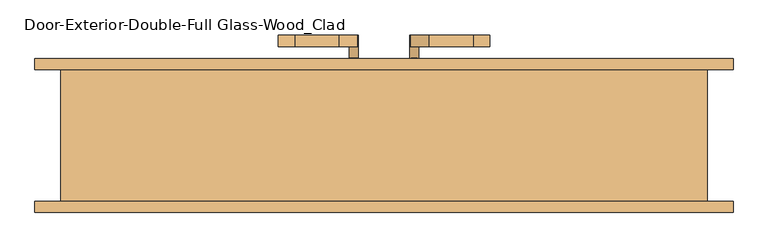
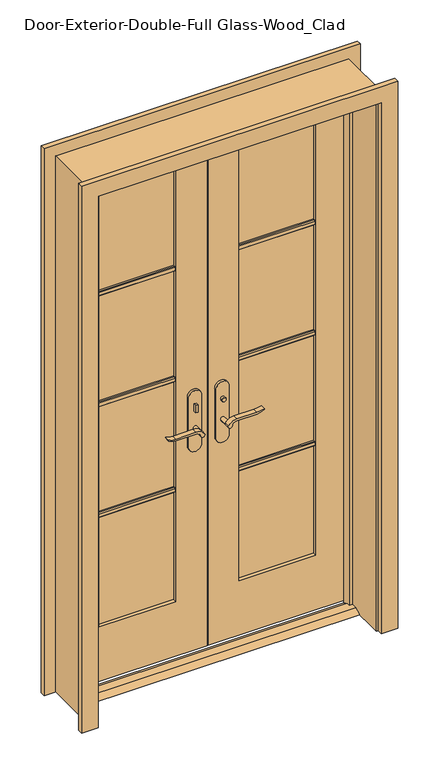
"""IFC4 building model written with IfcOpenShell, lengths in millimetres: door geometry, Door-Exterior-Double-Full Glass-Wood_Clad."""

from ifc_helpers import new_model, si_unit, point, frame, frame_2d, origin, place, context, project, spatial, polyline, circle_curve, trimmed, segment, composite_curve, outline, extrude, faceted_brep, source, transform, mapped, element, save


def door_exterior_double_full_glass_wood_clad_a9b2ee3b(model_context):
    return source(origin(), model_context, "Body", "SolidModel", [
        extrude(outline(polyline([(19.05, 12.7), (53.975, 12.7), (79.375, 0.0), (-6.35, 0.0), (19.05, 12.7)])), frame((-533.4, 0.0, 0.0), z_axis=(1.0, 0.0, 0.0), x_axis=(0.0, 1.0, 0.0)), (0.0, 0.0, 1.0), 1066.8),
        extrude(outline(polyline([(-47.4019111, 56.2), (-57.4019111, 56.2), (-57.4019111, 66.2), (-47.4019111, 66.2), (-47.4019111, 56.2)])), frame((0.0, 0.0, 981.9), z_axis=(0.0, 0.0, 1.0), x_axis=(1.0, 0.0, 0.0)), (0.0, 0.0, 1.0), 30.0),
        extrude(outline(composite_curve([segment(trimmed(circle_curve(frame_2d((996.9, -52.4019111)), 8.0), [point((996.9, -60.4019111))], [point((996.9, -44.4019111))], False, "CARTESIAN"), True, "CONTINUOUS"), segment(trimmed(circle_curve(frame_2d((996.9, -52.4019111)), 8.0), [point((996.9, -44.4019111))], [point((996.9, -60.4019111))], False, "CARTESIAN"), True, "CONTINUOUS")], self_intersect=False)), frame((0.0, 121.125, 0.0), z_axis=(0.0, 1.0, 0.0), x_axis=(0.0, 0.0, 1.0)), (0.0, 0.0, 1.0), 10.0),
        extrude(outline(composite_curve([segment(trimmed(circle_curve(frame_2d((897.1555521, -76.0694241)), 37.2832219), [point((919.0523287, -45.8937749))], [point((934.4, -77.7693445))], False, "CARTESIAN"), True, "CONTINUOUS"), segment(polyline([(934.4, -77.7693445), (934.4, -154.045502)]), True, "CONTINUOUS"), segment(trimmed(circle_curve(frame_2d((1017.6850638, -153.9791202)), 83.2850902), [point((934.4, -154.045502))], [point((939.4, -182.4019111))], True, "CARTESIAN"), True, "CONTINUOUS"), segment(polyline([(939.4, -182.4019111), (936.6135558, -182.4019111)]), True, "CONTINUOUS"), segment(trimmed(circle_curve(frame_2d((986.6709207, -150.4622499)), 59.3791355), [point((936.6135558, -182.4019111))], [point((927.4, -154.045502))], False, "CARTESIAN"), True, "CONTINUOUS"), segment(polyline([(927.4, -154.045502), (927.4, -77.7881013)]), True, "CONTINUOUS"), segment(trimmed(circle_curve(frame_2d((909.2738613, -77.7881013)), 18.1261387), [point((927.4, -77.7881013))], [point((914.4, -60.4019111))], True, "CARTESIAN"), True, "CONTINUOUS"), segment(trimmed(circle_curve(frame_2d((914.4, -52.4019111)), 8.0), [point((914.4, -60.4019111))], [point((919.0523287, -45.8937749))], False, "CARTESIAN"), True, "CONTINUOUS")], self_intersect=False)), frame((0.0, 16.2, 0.0), z_axis=(0.0, 1.0, 0.0), x_axis=(0.0, 0.0, 1.0)), (0.0, 0.0, 1.0), 20.0),
        extrude(outline(composite_curve([segment(trimmed(circle_curve(frame_2d((914.4, -52.4019111)), 8.0), [point((914.3999903, -60.4019111))], [point((919.0523287, -45.8937749))], False, "CARTESIAN"), True, "CONTINUOUS"), segment(trimmed(circle_curve(frame_2d((897.1555521, -76.0694241)), 37.2832219), [point((919.0523287, -45.8937749))], [point((934.4, -77.7693445))], False, "CARTESIAN"), True, "CONTINUOUS"), segment(polyline([(934.4, -77.7693445), (934.4, -154.045502)]), True, "CONTINUOUS"), segment(trimmed(circle_curve(frame_2d((1017.6850638, -153.9791202)), 83.2850902), [point((934.4, -154.045502))], [point((939.4, -182.4019111))], True, "CARTESIAN"), True, "CONTINUOUS"), segment(polyline([(939.4, -182.4019111), (936.6135558, -182.4019111)]), True, "CONTINUOUS"), segment(trimmed(circle_curve(frame_2d((986.6709207, -150.4622499)), 59.3791355), [point((936.6135558, -182.4019111))], [point((927.4, -154.045502))], False, "CARTESIAN"), True, "CONTINUOUS"), segment(polyline([(927.4, -154.045502), (927.4, -77.788099)]), True, "CONTINUOUS"), segment(trimmed(circle_curve(frame_2d((909.2738682, -77.788099)), 18.1261318), [point((927.4, -77.788099))], [point((914.3999903, -60.4019111))], True, "CARTESIAN"), True, "CONTINUOUS")], self_intersect=False)), frame((0.0, 151.125, 0.0), z_axis=(0.0, 1.0, 0.0), x_axis=(0.0, 0.0, 1.0)), (0.0, 0.0, 1.0), 20.0),
        extrude(outline(composite_curve([segment(trimmed(circle_curve(frame_2d((914.4, -52.4019111)), 8.0), [point((914.4, -60.4019111))], [point((914.4, -44.4019111))], False, "CARTESIAN"), True, "CONTINUOUS"), segment(trimmed(circle_curve(frame_2d((914.4, -52.4019111)), 8.0), [point((914.4, -44.4019111))], [point((914.4, -60.4019111))], False, "CARTESIAN"), True, "CONTINUOUS")], self_intersect=False)), frame((0.0, 36.2, 0.0), z_axis=(0.0, 1.0, 0.0), x_axis=(0.0, 0.0, 1.0)), (0.0, 0.0, 1.0), 30.0),
        extrude(outline(composite_curve([segment(trimmed(circle_curve(frame_2d((914.4, -52.4019111)), 8.0), [point((914.4, -60.4019111))], [point((914.4, -44.4019111))], False, "CARTESIAN"), True, "CONTINUOUS"), segment(trimmed(circle_curve(frame_2d((914.4, -52.4019111)), 8.0), [point((914.4, -44.4019111))], [point((914.4, -60.4019111))], False, "CARTESIAN"), True, "CONTINUOUS")], self_intersect=False)), frame((0.0, 121.125, 0.0), z_axis=(0.0, 1.0, 0.0), x_axis=(0.0, 0.0, 1.0)), (0.0, 0.0, 1.0), 30.0),
        extrude(outline(composite_curve([segment(polyline([(844.4, -27.4019111), (1039.4, -27.4019111)]), True, "CONTINUOUS"), segment(trimmed(circle_curve(frame_2d((1039.4, -52.4019111)), 25.0), [point((1039.4, -27.4019111))], [point((1039.4, -77.4019111))], False, "CARTESIAN"), True, "CONTINUOUS"), segment(polyline([(1039.4, -77.4019111), (844.4, -77.4019111)]), True, "CONTINUOUS"), segment(trimmed(circle_curve(frame_2d((844.4, -52.4019111)), 25.0), [point((844.4, -77.4019111))], [point((844.4, -27.4019111))], False, "CARTESIAN"), True, "CONTINUOUS")], self_intersect=False)), frame((0.0, 66.2, 0.0), z_axis=(0.0, 1.0, 0.0), x_axis=(0.0, 0.0, 1.0)), (0.0, 0.0, 1.0), 10.0),
        extrude(outline(composite_curve([segment(polyline([(844.4, -27.4019111), (1039.4, -27.4019111)]), True, "CONTINUOUS"), segment(trimmed(circle_curve(frame_2d((1039.4, -52.4019111)), 25.0), [point((1039.4, -27.4019111))], [point((1039.4, -77.4019111))], False, "CARTESIAN"), True, "CONTINUOUS"), segment(polyline([(1039.4, -77.4019111), (844.4, -77.4019111)]), True, "CONTINUOUS"), segment(trimmed(circle_curve(frame_2d((844.4, -52.4019111)), 25.0), [point((844.4, -77.4019111))], [point((844.4, -27.4019111))], False, "CARTESIAN"), True, "CONTINUOUS")], self_intersect=False)), frame((0.0, 111.125, 0.0), z_axis=(0.0, 1.0, 0.0), x_axis=(0.0, 0.0, 1.0)), (0.0, 0.0, 1.0), 10.0),
        extrude(outline(polyline([(47.3875, 131.125), (57.3875, 131.125), (57.3875, 121.125), (47.3875, 121.125), (47.3875, 131.125)])), frame((0.0, 0.0, 981.9), z_axis=(0.0, 0.0, 1.0), x_axis=(1.0, 0.0, 0.0)), (0.0, 0.0, 1.0), 30.0),
        extrude(outline(composite_curve([segment(trimmed(circle_curve(frame_2d((996.9, 52.3875)), 8.0), [point((996.9, 60.3875))], [point((996.9, 44.3875))], False, "CARTESIAN"), True, "CONTINUOUS"), segment(trimmed(circle_curve(frame_2d((996.9, 52.3875)), 8.0), [point((996.9, 44.3875))], [point((996.9, 60.3875))], False, "CARTESIAN"), True, "CONTINUOUS")], self_intersect=False)), frame((0.0, 56.2, 0.0), z_axis=(0.0, 1.0, 0.0), x_axis=(0.0, 0.0, 1.0)), (0.0, 0.0, 1.0), 10.0),
        extrude(outline(composite_curve([segment(trimmed(circle_curve(frame_2d((914.4, 52.3875)), 8.0), [point((919.0523287, 45.8793637))], [point((914.4, 60.3875))], False, "CARTESIAN"), True, "CONTINUOUS"), segment(trimmed(circle_curve(frame_2d((909.2738613, 77.7736901)), 18.1261387), [point((914.4, 60.3875))], [point((927.4, 77.7736901))], True, "CARTESIAN"), True, "CONTINUOUS"), segment(polyline([(927.4, 77.7736901), (927.4, 154.0310909)]), True, "CONTINUOUS"), segment(trimmed(circle_curve(frame_2d((986.6709207, 150.4478388)), 59.3791355), [point((927.4, 154.0310909))], [point((936.6135558, 182.3875))], False, "CARTESIAN"), True, "CONTINUOUS"), segment(polyline([(936.6135558, 182.3875), (939.4, 182.3875)]), True, "CONTINUOUS"), segment(trimmed(circle_curve(frame_2d((1017.6850638, 153.9647091)), 83.2850902), [point((939.4, 182.3875))], [point((934.4, 154.0310909))], True, "CARTESIAN"), True, "CONTINUOUS"), segment(polyline([(934.4, 154.0310909), (934.4, 77.7549333)]), True, "CONTINUOUS"), segment(trimmed(circle_curve(frame_2d((897.1555521, 76.0550129)), 37.2832219), [point((934.4, 77.7549333))], [point((919.0523287, 45.8793637))], False, "CARTESIAN"), True, "CONTINUOUS")], self_intersect=False)), frame((0.0, 151.125, 0.0), z_axis=(0.0, 1.0, 0.0), x_axis=(0.0, 0.0, 1.0)), (0.0, 0.0, 1.0), 20.0),
        extrude(outline(composite_curve([segment(trimmed(circle_curve(frame_2d((909.2738682, 77.7736878)), 18.1261318), [point((914.3999903, 60.3875))], [point((927.4, 77.7736878))], True, "CARTESIAN"), True, "CONTINUOUS"), segment(polyline([(927.4, 77.7736878), (927.4, 154.0310909)]), True, "CONTINUOUS"), segment(trimmed(circle_curve(frame_2d((986.6709207, 150.4478388)), 59.3791355), [point((927.4, 154.0310909))], [point((936.6135558, 182.3875))], False, "CARTESIAN"), True, "CONTINUOUS"), segment(polyline([(936.6135558, 182.3875), (939.4, 182.3875)]), True, "CONTINUOUS"), segment(trimmed(circle_curve(frame_2d((1017.6850638, 153.9647091)), 83.2850902), [point((939.4, 182.3875))], [point((934.4, 154.0310909))], True, "CARTESIAN"), True, "CONTINUOUS"), segment(polyline([(934.4, 154.0310909), (934.4, 77.7549333)]), True, "CONTINUOUS"), segment(trimmed(circle_curve(frame_2d((897.1555521, 76.0550129)), 37.2832219), [point((934.4, 77.7549333))], [point((919.0523287, 45.8793637))], False, "CARTESIAN"), True, "CONTINUOUS"), segment(trimmed(circle_curve(frame_2d((914.4, 52.3875)), 8.0), [point((919.0523287, 45.8793637))], [point((914.3999903, 60.3875))], False, "CARTESIAN"), True, "CONTINUOUS")], self_intersect=False)), frame((0.0, 16.2, 0.0), z_axis=(0.0, 1.0, 0.0), x_axis=(0.0, 0.0, 1.0)), (0.0, 0.0, 1.0), 20.0),
        extrude(outline(composite_curve([segment(trimmed(circle_curve(frame_2d((914.4, 52.3875)), 8.0), [point((914.4, 60.3875))], [point((914.4, 44.3875))], False, "CARTESIAN"), True, "CONTINUOUS"), segment(trimmed(circle_curve(frame_2d((914.4, 52.3875)), 8.0), [point((914.4, 44.3875))], [point((914.4, 60.3875))], False, "CARTESIAN"), True, "CONTINUOUS")], self_intersect=False)), frame((0.0, 121.125, 0.0), z_axis=(0.0, 1.0, 0.0), x_axis=(0.0, 0.0, 1.0)), (0.0, 0.0, 1.0), 30.0),
        extrude(outline(composite_curve([segment(trimmed(circle_curve(frame_2d((914.4, 52.3875)), 8.0), [point((914.4, 60.3875))], [point((914.4, 44.3875))], False, "CARTESIAN"), True, "CONTINUOUS"), segment(trimmed(circle_curve(frame_2d((914.4, 52.3875)), 8.0), [point((914.4, 44.3875))], [point((914.4, 60.3875))], False, "CARTESIAN"), True, "CONTINUOUS")], self_intersect=False)), frame((0.0, 36.2, 0.0), z_axis=(0.0, 1.0, 0.0), x_axis=(0.0, 0.0, 1.0)), (0.0, 0.0, 1.0), 30.0),
        extrude(outline(composite_curve([segment(trimmed(circle_curve(frame_2d((844.4, 52.3875)), 25.0), [point((844.4, 27.3875))], [point((844.4, 77.3875))], False, "CARTESIAN"), True, "CONTINUOUS"), segment(polyline([(844.4, 77.3875), (1039.4, 77.3875)]), True, "CONTINUOUS"), segment(trimmed(circle_curve(frame_2d((1039.4, 52.3875)), 25.0), [point((1039.4, 77.3875))], [point((1039.4, 27.3875))], False, "CARTESIAN"), True, "CONTINUOUS"), segment(polyline([(1039.4, 27.3875), (844.4, 27.3875)]), True, "CONTINUOUS")], self_intersect=False)), frame((0.0, 111.125, 0.0), z_axis=(0.0, 1.0, 0.0), x_axis=(0.0, 0.0, 1.0)), (0.0, 0.0, 1.0), 10.0),
        extrude(outline(composite_curve([segment(trimmed(circle_curve(frame_2d((844.4, 52.3875)), 25.0), [point((844.4, 27.3875))], [point((844.4, 77.3875))], False, "CARTESIAN"), True, "CONTINUOUS"), segment(polyline([(844.4, 77.3875), (1039.4, 77.3875)]), True, "CONTINUOUS"), segment(trimmed(circle_curve(frame_2d((1039.4, 52.3875)), 25.0), [point((1039.4, 77.3875))], [point((1039.4, 27.3875))], False, "CARTESIAN"), True, "CONTINUOUS"), segment(polyline([(1039.4, 27.3875), (844.4, 27.3875)]), True, "CONTINUOUS")], self_intersect=False)), frame((0.0, 66.2, 0.0), z_axis=(0.0, 1.0, 0.0), x_axis=(0.0, 0.0, 1.0)), (0.0, 0.0, 1.0), 10.0),
        extrude(outline(polyline([(90.17, 1578.371875), (90.17, 1559.321875), (83.82, 1559.321875), (80.645, 1562.496875), (80.645, 1575.196875), (83.82, 1578.371875), (90.17, 1578.371875)])), frame((120.65, 0.0, 0.0), z_axis=(1.0, 0.0, 0.0), x_axis=(0.0, 1.0, 0.0)), (0.0, 0.0, 1.0), 292.1),
        extrude(outline(polyline([(90.17, 1132.68125), (90.17, 1113.63125), (83.82, 1113.63125), (80.645, 1116.80625), (80.645, 1129.50625), (83.82, 1132.68125), (90.17, 1132.68125)])), frame((120.65, 0.0, 0.0), z_axis=(1.0, 0.0, 0.0), x_axis=(0.0, 1.0, 0.0)), (0.0, 0.0, 1.0), 292.1),
        extrude(outline(polyline([(90.17, 686.990625), (90.17, 667.940625), (83.82, 667.940625), (80.645, 671.115625), (80.645, 683.815625), (83.82, 686.990625), (90.17, 686.990625)])), frame((120.65, 0.0, 0.0), z_axis=(1.0, 0.0, 0.0), x_axis=(0.0, 1.0, 0.0)), (0.0, 0.0, 1.0), 292.1),
        extrude(outline(polyline([(97.155, 1578.371875), (103.505, 1578.371875), (106.68, 1575.196875), (106.68, 1562.496875), (103.505, 1559.321875), (97.155, 1559.321875), (97.155, 1578.371875)])), frame((-412.75, 0.0, 0.0), z_axis=(1.0, 0.0, 0.0), x_axis=(0.0, 1.0, 0.0)), (0.0, 0.0, 1.0), 292.1),
        extrude(outline(polyline([(97.155, 1132.68125), (103.505, 1132.68125), (106.68, 1129.50625), (106.68, 1116.80625), (103.505, 1113.63125), (97.155, 1113.63125), (97.155, 1132.68125)])), frame((-412.75, 0.0, 0.0), z_axis=(1.0, 0.0, 0.0), x_axis=(0.0, 1.0, 0.0)), (0.0, 0.0, 1.0), 292.1),
        extrude(outline(polyline([(97.155, 686.990625), (103.505, 686.990625), (106.68, 683.815625), (106.68, 671.115625), (103.505, 667.940625), (97.155, 667.940625), (97.155, 686.990625)])), frame((-412.75, 0.0, 0.0), z_axis=(1.0, 0.0, 0.0), x_axis=(0.0, 1.0, 0.0)), (0.0, 0.0, 1.0), 292.1),
        extrude(outline(polyline([(97.155, 1578.371875), (103.505, 1578.371875), (106.68, 1575.196875), (106.68, 1562.496875), (103.505, 1559.321875), (97.155, 1559.321875), (97.155, 1578.371875)])), frame((120.65, 0.0, 0.0), z_axis=(1.0, 0.0, 0.0), x_axis=(0.0, 1.0, 0.0)), (0.0, 0.0, 1.0), 292.1),
        extrude(outline(polyline([(97.155, 1132.68125), (103.505, 1132.68125), (106.68, 1129.50625), (106.68, 1116.80625), (103.505, 1113.63125), (97.155, 1113.63125), (97.155, 1132.68125)])), frame((120.65, 0.0, 0.0), z_axis=(1.0, 0.0, 0.0), x_axis=(0.0, 1.0, 0.0)), (0.0, 0.0, 1.0), 292.1),
        extrude(outline(polyline([(97.155, 686.990625), (103.505, 686.990625), (106.68, 683.815625), (106.68, 671.115625), (103.505, 667.940625), (97.155, 667.940625), (97.155, 686.990625)])), frame((120.65, 0.0, 0.0), z_axis=(1.0, 0.0, 0.0), x_axis=(0.0, 1.0, 0.0)), (0.0, 0.0, 1.0), 292.1),
        extrude(outline(polyline([(90.17, 1578.371875), (90.17, 1559.321875), (83.82, 1559.321875), (80.645, 1562.496875), (80.645, 1575.196875), (83.82, 1578.371875), (90.17, 1578.371875)])), frame((-412.75, 0.0, 0.0), z_axis=(1.0, 0.0, 0.0), x_axis=(0.0, 1.0, 0.0)), (0.0, 0.0, 1.0), 292.1),
        extrude(outline(polyline([(90.17, 1132.68125), (90.17, 1113.63125), (83.82, 1113.63125), (80.645, 1116.80625), (80.645, 1129.50625), (83.82, 1132.68125), (90.17, 1132.68125)])), frame((-412.75, 0.0, 0.0), z_axis=(1.0, 0.0, 0.0), x_axis=(0.0, 1.0, 0.0)), (0.0, 0.0, 1.0), 292.1),
        extrude(outline(polyline([(90.17, 686.990625), (90.17, 667.940625), (83.82, 667.940625), (80.645, 671.115625), (80.645, 683.815625), (83.82, 686.990625), (90.17, 686.990625)])), frame((-412.75, 0.0, 0.0), z_axis=(1.0, 0.0, 0.0), x_axis=(0.0, 1.0, 0.0)), (0.0, 0.0, 1.0), 292.1),
        extrude(outline(polyline([(0.0, 539.75), (0.0, 603.25), (2203.45, 603.25), (2203.45, -603.25), (0.0, -603.25), (0.0, -539.75), (2139.95, -539.75), (2139.95, 539.75), (0.0, 539.75)])), frame((0.0, -136.525, 0.0), z_axis=(0.0, 1.0, 0.0), x_axis=(0.0, 0.0, 1.0)), (0.0, 0.0, 1.0), 19.05),
        extrude(outline(polyline([(0.0, 539.75), (0.0, 603.25), (2203.45, 603.25), (2203.45, -603.25), (0.0, -603.25), (0.0, -539.75), (2139.95, -539.75), (2139.95, 539.75), (0.0, 539.75)])), frame((0.0, 111.125, 0.0), z_axis=(0.0, 1.0, 0.0), x_axis=(0.0, 0.0, 1.0)), (0.0, 0.0, 1.0), 19.05),
        faceted_brep([(558.8, 111.125, 0.0), (558.8, -117.475, 0.0), (533.4, -117.475, 0.0), (533.4, 41.275, 0.0), (520.7, 41.275, 0.0), (520.7, 76.2, 0.0), (533.4, 76.2, 0.0), (533.4, 111.125, 0.0), (558.8, 111.125, 2159.0), (558.8, -117.475, 2159.0), (-558.8, -117.475, 2159.0), (-558.8, -117.475, 0.0), (-533.4, -117.475, 0.0), (-533.4, -117.475, 2133.6), (533.4, -117.475, 2133.6), (533.4, 41.275, 2133.6), (-533.4, 41.275, 2133.6), (-533.4, 41.275, 0.0), (-520.7, 41.275, 0.0), (-520.7, 41.275, 2120.9), (520.7, 41.275, 2120.9), (520.7, 76.2, 2120.9), (1.5875, 76.2, 2120.9), (-1.6019111, 76.2, 2120.9), (-520.7, 76.2, 2120.9), (-520.7, 76.2, 0.0), (-533.4, 76.2, 0.0), (-533.4, 76.2, 2133.6), (-1.6019111, 76.2, 2133.6), (1.5875, 76.2, 2133.6), (533.4, 76.2, 2133.6), (533.4, 111.125, 2133.6), (1.5875, 111.125, 2133.6), (-1.6019111, 111.125, 2133.6), (-533.4, 111.125, 2133.6), (-533.4, 111.125, 0.0), (-558.8, 111.125, 0.0), (-558.8, 111.125, 2159.0)], [[[0, 1, 2, 3, 4, 5, 6, 7]], [[1, 0, 8, 9]], [[2, 1, 9, 10, 11, 12, 13, 14]], [[3, 2, 14, 15]], [[4, 3, 15, 16, 17, 18, 19, 20]], [[5, 4, 20, 21]], [[6, 5, 21, 22, 23, 24, 25, 26, 27, 28, 29, 30]], [[7, 6, 30, 31]], [[0, 7, 31, 32, 33, 34, 35, 36, 37, 8]], [[9, 8, 37, 10]], [[14, 13, 16, 15]], [[20, 19, 24, 23, 22, 21]], [[31, 30, 29, 28, 27, 34, 33, 32]], [[12, 11, 36, 35, 26, 25, 18, 17]], [[11, 10, 37, 36]], [[13, 12, 17, 16]], [[19, 18, 25, 24]], [[27, 26, 35, 34]]]),
        extrude(outline(polyline([(12.7, 533.4), (2133.6, 533.4), (2133.6, 1.5875), (12.7, 1.5875), (12.7, 533.4)]), holes=[polyline([(2014.5375, 120.65), (2014.5375, 412.75), (231.775, 412.75), (231.775, 120.65), (2014.5375, 120.65)])]), frame((0.0, 76.2, 0.0), z_axis=(0.0, 1.0, 0.0), x_axis=(0.0, 0.0, 1.0)), (0.0, 0.0, 1.0), 34.925),
        extrude(outline(polyline([(2133.6, -533.4), (12.7, -533.4), (12.7, -1.6019111), (2133.6, -1.6019111), (2133.6, -533.4)]), holes=[polyline([(231.775, -412.75), (2014.5375, -412.75), (2014.5375, -120.65), (231.775, -120.65), (231.775, -412.75)])]), frame((0.0, 76.2, 0.0), z_axis=(0.0, 1.0, 0.0), x_axis=(0.0, 0.0, 1.0)), (0.0, 0.0, 1.0), 34.925),
        extrude(outline(polyline([(412.75, 90.17), (120.65, 90.17), (120.65, 97.155), (412.75, 97.155), (412.75, 90.17)])), frame((0.0, 0.0, 231.775), z_axis=(0.0, 0.0, 1.0), x_axis=(1.0, 0.0, 0.0)), (0.0, 0.0, 1.0), 1782.7625),
        extrude(outline(polyline([(-120.65, 90.17), (-412.75, 90.17), (-412.75, 97.155), (-120.65, 97.155), (-120.65, 90.17)])), frame((0.0, 0.0, 231.775), z_axis=(0.0, 0.0, 1.0), x_axis=(1.0, 0.0, 0.0)), (0.0, 0.0, 1.0), 1782.7625),
    ])


if __name__ == "__main__":
    model = new_model("IFC4")
    model_context = context("Model", 3, world=origin())
    ifc_project = project(units=[si_unit("LENGTHUNIT", "METRE", prefix="MILLI")], contexts=[model_context])
    site = spatial("IfcSite", under=ifc_project)
    building = spatial("IfcBuilding", under=site)
    placement = place(None, origin())
    door_exterior_double_full_glass_wood_clad_shape = door_exterior_double_full_glass_wood_clad_a9b2ee3b(model_context)
    element("IfcDoor", 1, ObjectType="Door-Exterior-Double-Full Glass-Wood_Clad", at=placement, inside=building, context=model_context, shape_type="MappedRepresentation", body=[
        mapped(door_exterior_double_full_glass_wood_clad_shape, transform((0.0, 0.0, 0.0), x_axis=(1.0, 0.0, 0.0), y_axis=(0.0, 1.0, 0.0), z_axis=(0.0, 0.0, 1.0))),
    ])
    save(model, "model.ifc")

# Revit data of these elements
# Type "Door-Exterior-Double-Full Glass-Wood_Clad"
#   Type Mark = "9"
#   Assembly Code = "B2030100"
#   Analytic Construction = "French door, wood frame with double glass"
#   Top Rail = 0' - 4 11/16"
#   Threshold Offset [instance default] = 0' - 0 1/2"
#   Thickness = 0' - 1 3/8"
#   Thermal Resistance (R) = 1.9158 (h·ft²·°F)/BTU
#   Swing Angle [instance default] = 90.00°
#   Stiles = 0' - 4 3/4"
#   Rough Width = 3' - 8"
#   Rough Height = 7' - 1"
#   Panel Width = 1' - 9"
#   Door Offset [instance default] = 0' - 0"
#   Height = 7' - 0"
#   Width = 3' - 6"
#   Heat Transfer Coefficient (U) = 0.5220 BTU/(h·ft²·°F)
#   Bottom Rail = 0' - 9 1/8"
#   Exterior Trim [instance default] = yes
#   Threshold [instance default] = yes
#   Show Grill [instance default] = yes
#   Function = 1
#   Trim Material = Cherry
#   Threshold Material = Cherry
#   Panel Material = Cherry
#   Glazing = Glass
#   Frame Material = Cherry
#   Door Handle Material = Aluminum
#   Visual Light Transmittance = 0
#   Solar Heat Gain Coefficient = 0
#   Wall Closure = (empty or 0)
#   Construction Type = (empty or 0)
# Element 1 (IfcDoor, "Door-Exterior-Double-Full Glass-Wood_Clad")
#   Materials on its faces: "Cherry", "Aluminum", "Glass"
# Materials
#   "Cherry": class "Wood", colour RGB 226 177 128, transparency 0, Description = "Prunus Serotina", Cost = 0
#   "Glass": class "Glass", colour RGB 0 128 192, transparency 0.75, Description = "Soda Lime Glass", Cost = 0
#   "Aluminum": class "Metal", colour RGB 247 247 247, transparency 0, Description = "Aluminum 6061", Cost = 0
